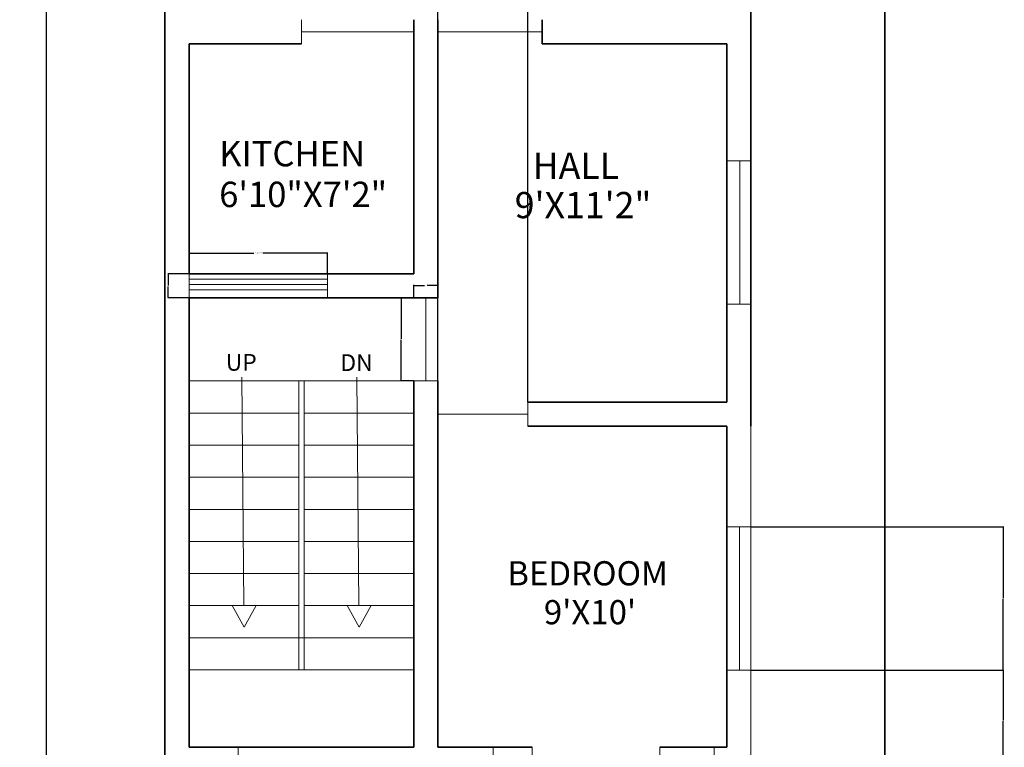
# Model space of a CAD drawing. Units: feet. Extents: x 2100 to 2836, y 2433 to 3396.
# Tile 6 of 12: x 2468 to 2836, y 2634 to 2906. Entities that reach past the tile are written whole.
import ezdxf

# ---------------------------------------------------------------- set-up
doc = ezdxf.new("R2010")
doc.units = ezdxf.units.FT
for name, color, linetype, lineweight in [('A-ANNO-DIMS', 2, 'Continuous', 18), ('A-ANNO-SYMB', 2, 'Continuous', 13), ('A-ANNO-TEXT', 7, 'Continuous', 18), ('A-ANNO-TTLB', 7, 'Continuous', 35), ('A-AREA-IDEN', 7, 'Continuous', 18), ('A-DOOR', 3, 'Continuous', 18), ('A-FLOR-STRS', 2, 'Continuous', 20), ('A-GLAZ', 4, 'Continuous', 18), ('A-WALL', 7, 'Continuous', 35), ('C-PROP', 8, 'Continuous', 18)]:
    doc.layers.add(name, color=color, linetype=linetype, lineweight=lineweight)
doc.styles.get("Standard").update_dxf_attribs({"font": 'arial.ttf'})
doc.dimstyles.get("Standard").update_dxf_attribs({"dimtxt": 0.18, "dimasz": 0.18, "dimexe": 0.18, "dimexo": 0.0625, "dimgap": 0.09, "dimtad": 0, "dimtih": 1, "dimtoh": 1, "dimdec": 4, "dimzin": 0, "dimdsep": 46, "dimtxsty": 'Standard', "dimcen": 0.09, "dimadec": 0, "dimazin": 0, "dimtfac": 1, "dimtdec": 4, "dimtofl": 0, "dimtmove": 0, "dimatfit": 3, "dimfxl": 1, "dimtolj": 1, "dimtzin": 0, "dimarcsym": 0})

# ---------------------------------------------------------------- blocks, each defined once
blk = doc.blocks.new('STAIR-RETURN-FLIGHT')
for p, q in [((84, 108), (0, 108)), ((41, 108), (41, 0)), ((43, 108), (43, 0)), ((41, 96), (0, 96)), ((84, 96), (43, 96)), ((41, 84), (0, 84)), ((84, 84), (43, 84)), ((41, 72), (0, 72)), ((84, 72), (43, 72)), ((41, 60), (0, 60)), ((84, 60), (43, 60)), ((41, 48), (0, 48)), ((84, 48), (43, 48)), ((41, 36), (0, 36)), ((84, 36), (43, 36)), ((41, 24), (0, 24)), ((84, 24), (43, 24)), ((84, 12), (0, 12)), ((84, 0), (0, 0))]:
    blk.add_line(p, q)
blk = doc.blocks.new('STAIR-DIRECTION')
for p, q in [((3.63, 93.38), (4.37, 8)), ((4.44, 0), (0, 8)), ((4.44, 0), (8.95, 8))]:
    blk.add_line(p, q)
blk = doc.blocks.new('WIN-KITCHEN')
for p, q in [((0, 9), (0, 0)), ((51.75, 9), (51.75, 0)), ((51.75, 7), (0, 7)), ((51.75, 5), (0, 5)), ((51.75, 3), (0, 3))]:
    blk.add_line(p, q)
blk = doc.blocks.new('DOOR-STAIR-HALL')
for p, q in [((4.5, 0), (4.5, 31.05)), ((9, 0), (0, 0))]:
    blk.add_line(p, q)
blk = doc.blocks.new('DOOR-PASSAGE')
for p, q in [((42, 0), (42, 9)), ((42, 4.5), (0, 4.5))]:
    blk.add_line(p, q)
blk = doc.blocks.new('DOOR-SLIDING-ENTRY')
for p, q in [((0, 9), (0, 0)), ((14.54, 9), (14.54, 0)), ((62.31, 9), (62.31, 0)), ((82.55, 9), (82.55, 0)), ((0, 4.5), (82.55, 4.5))]:
    blk.add_line(p, q)
blk = doc.blocks.new('*D22')
at = {"layer": 'A-ANNO-DIMS', "color": 0, "lineweight": -2, "transparency": 16777216}
for p, q in [((2530.95, 2810.87), (2530.95, 2818.75)), ((2531.13, 2818.57), (2555.12, 2818.57)), ((2582.52, 2818.57), (2558.52, 2818.57)), ((2582.7, 2810.87), (2582.7, 2818.75))]:
    blk.add_line(p, q, dxfattribs=at)
at = {"layer": 'A-ANNO-DIMS', "color": 0, "transparency": 16777216}
for points in [[(2531.13, 2818.6), (2531.13, 2818.54), (2530.95, 2818.57)], [(2582.52, 2818.6), (2582.52, 2818.54), (2582.7, 2818.57)]]:
    blk.add_solid(points, dxfattribs=at)
at = {"layer": 'Defpoints', "color": 0, "transparency": 16777216}
for p in [(2582.7, 2818.57), (2530.95, 2810.8), (2582.7, 2810.8)]:
    blk.add_point(p, dxfattribs=at)
at = {"layer": 'A-ANNO-DIMS', "color": 0, "transparency": 16777216, "insert": (2556.82, 2818.57), "char_height": 0.18, "attachment_point": 5}
blk.add_mtext('\\A1;KITCHEN WINDOW 52 TYP.', dxfattribs=at)
blk = doc.blocks.new('*D23')
at = {"layer": 'A-ANNO-DIMS', "color": 0, "lineweight": -2, "transparency": 16777216}
for p, q in [((2530.89, 2810.8), (2523.01, 2810.8)), ((2523.19, 2810.62), (2523.19, 2806.48)), ((2523.19, 2801.98), (2523.19, 2806.12)), ((2530.89, 2801.8), (2523.01, 2801.8))]:
    blk.add_line(p, q, dxfattribs=at)
at = {"layer": 'A-ANNO-DIMS', "color": 0, "transparency": 16777216}
for points in [[(2523.16, 2810.62), (2523.22, 2810.62), (2523.19, 2810.8)], [(2523.16, 2801.98), (2523.22, 2801.98), (2523.19, 2801.8)]]:
    blk.add_solid(points, dxfattribs=at)
at = {"layer": 'Defpoints', "color": 0, "transparency": 16777216}
for p in [(2523.19, 2810.8), (2530.95, 2810.8), (2530.95, 2801.8)]:
    blk.add_point(p, dxfattribs=at)
at = {"layer": 'A-ANNO-DIMS', "color": 0, "transparency": 16777216, "insert": (2523.19, 2806.3), "char_height": 0.18, "attachment_point": 5}
blk.add_mtext('\\A1;9 TYP.', dxfattribs=at)
blk = doc.blocks.new('*D36')
at = {"layer": 'A-ANNO-DIMS', "color": 0, "lineweight": -2, "transparency": 16777216}
for p, q in [((2614.89, 2801.8), (2610.11, 2801.8)), ((2610.29, 2801.62), (2610.29, 2786.46)), ((2610.29, 2770.94), (2610.29, 2786.1)), ((2614.89, 2770.76), (2610.11, 2770.76))]:
    blk.add_line(p, q, dxfattribs=at)
at = {"layer": 'A-ANNO-DIMS', "color": 0, "transparency": 16777216}
for points in [[(2610.26, 2801.62), (2610.32, 2801.62), (2610.29, 2801.8)], [(2610.26, 2770.94), (2610.32, 2770.94), (2610.29, 2770.76)]]:
    blk.add_solid(points, dxfattribs=at)
at = {"layer": 'Defpoints', "color": 0, "transparency": 16777216}
for p in [(2610.29, 2801.8), (2614.95, 2801.8), (2614.95, 2770.76)]:
    blk.add_point(p, dxfattribs=at)
at = {"layer": 'A-ANNO-DIMS', "color": 0, "transparency": 16777216, "insert": (2610.29, 2786.28), "char_height": 0.18, "attachment_point": 5}
blk.add_mtext('\\A1;HALL DOOR 31 TYP.', dxfattribs=at)
blk = doc.blocks.new('*D37')
at = {"layer": 'A-ANNO-DIMS', "color": 0, "lineweight": -2, "transparency": 16777216}
for p, q in [((2614.95, 2801.87), (2614.95, 2806.64)), ((2615.13, 2806.46), (2618.99, 2806.46)), ((2623.77, 2806.46), (2619.91, 2806.46)), ((2623.95, 2801.87), (2623.95, 2806.64))]:
    blk.add_line(p, q, dxfattribs=at)
at = {"layer": 'A-ANNO-DIMS', "color": 0, "transparency": 16777216}
for points in [[(2615.13, 2806.49), (2615.13, 2806.43), (2614.95, 2806.46)], [(2623.77, 2806.49), (2623.77, 2806.43), (2623.95, 2806.46)]]:
    blk.add_solid(points, dxfattribs=at)
at = {"layer": 'Defpoints', "color": 0, "transparency": 16777216}
for p in [(2623.95, 2806.46), (2614.95, 2801.8), (2623.95, 2801.8)]:
    blk.add_point(p, dxfattribs=at)
at = {"layer": 'A-ANNO-DIMS', "color": 0, "transparency": 16777216, "insert": (2619.45, 2806.46), "char_height": 0.18, "attachment_point": 5}
blk.add_mtext('\\A1;9 TYP.', dxfattribs=at)
blk = doc.blocks.new('*D43')
at = {"layer": 'A-ANNO-DIMS', "color": 0, "lineweight": -2, "transparency": 16777216}
for p, q in [((2521.89, 3321.8), (2477.52, 3321.8)), ((2477.7, 3321.62), (2477.7, 2929.96)), ((2477.7, 2537.94), (2477.7, 2929.6)), ((2521.89, 2537.76), (2477.52, 2537.76))]:
    blk.add_line(p, q, dxfattribs=at)
at = {"layer": 'A-ANNO-DIMS', "color": 0, "transparency": 16777216}
for points in [[(2477.67, 3321.62), (2477.73, 3321.62), (2477.7, 3321.8)], [(2477.67, 2537.94), (2477.73, 2537.94), (2477.7, 2537.76)]]:
    blk.add_solid(points, dxfattribs=at)
at = {"layer": 'Defpoints', "color": 0, "transparency": 16777216}
for p in [(2477.7, 3321.8), (2521.95, 3321.8), (2521.95, 2537.76)]:
    blk.add_point(p, dxfattribs=at)
at = {"layer": 'A-ANNO-DIMS', "color": 0, "transparency": 16777216, "insert": (2477.7, 2929.78), "char_height": 0.18, "attachment_point": 5}
blk.add_mtext('\\A1;784', dxfattribs=at)
blk = doc.blocks.new('*D57')
at = {"layer": 'A-ANNO-DIMS', "color": 0, "lineweight": -2, "transparency": 16777216}
for p, q in [((2741.01, 2662.65), (2835.49, 2662.65)), ((2835.31, 2662.47), (2835.31, 2643.91)), ((2835.31, 2624.98), (2835.31, 2643.54)), ((2741.01, 2624.8), (2835.49, 2624.8))]:
    blk.add_line(p, q, dxfattribs=at)
at = {"layer": 'A-ANNO-DIMS', "color": 0, "transparency": 16777216}
for points in [[(2835.28, 2662.47), (2835.34, 2662.47), (2835.31, 2662.65)], [(2835.28, 2624.98), (2835.34, 2624.98), (2835.31, 2624.8)]]:
    blk.add_solid(points, dxfattribs=at)
at = {"layer": 'Defpoints', "color": 0, "transparency": 16777216}
for p in [(2740.95, 2662.65), (2835.31, 2662.65), (2740.95, 2624.8)]:
    blk.add_point(p, dxfattribs=at)
at = {"layer": 'A-ANNO-DIMS', "color": 0, "transparency": 16777216, "insert": (2835.31, 2643.73), "char_height": 0.18, "attachment_point": 5}
blk.add_mtext('\\A1;37.845', dxfattribs=at)
blk = doc.blocks.new('*D58')
at = {"layer": 'A-ANNO-DIMS', "color": 0, "lineweight": -2, "transparency": 16777216}
for p, q in [((2741.01, 2716.27), (2835.49, 2716.27)), ((2835.31, 2716.09), (2835.31, 2689.64)), ((2835.31, 2662.83), (2835.31, 2689.28)), ((2741.01, 2662.65), (2835.49, 2662.65))]:
    blk.add_line(p, q, dxfattribs=at)
at = {"layer": 'A-ANNO-DIMS', "color": 0, "transparency": 16777216}
for points in [[(2835.28, 2716.09), (2835.34, 2716.09), (2835.31, 2716.27)], [(2835.28, 2662.83), (2835.34, 2662.83), (2835.31, 2662.65)]]:
    blk.add_solid(points, dxfattribs=at)
at = {"layer": 'Defpoints', "color": 0, "transparency": 16777216}
for p in [(2740.95, 2716.27), (2835.31, 2716.27), (2740.95, 2662.65)]:
    blk.add_point(p, dxfattribs=at)
at = {"layer": 'A-ANNO-DIMS', "color": 0, "transparency": 16777216, "insert": (2835.31, 2689.46), "char_height": 0.18, "attachment_point": 5}
blk.add_mtext('\\A1;53.62', dxfattribs=at)
blk = doc.blocks.new('*D62')
at = {"layer": 'A-ANNO-DIMS', "color": 0, "lineweight": -2, "transparency": 16777216}
for p, q in [((2623.95, 2762.87), (2623.95, 3396.05)), ((2624.13, 3395.87), (2640.32, 3395.87)), ((2657.43, 3395.87), (2641.24, 3395.87)), ((2657.61, 2762.87), (2657.61, 3396.05))]:
    blk.add_line(p, q, dxfattribs=at)
at = {"layer": 'A-ANNO-DIMS', "color": 0, "transparency": 16777216}
for points in [[(2624.13, 3395.9), (2624.13, 3395.84), (2623.95, 3395.87)], [(2657.43, 3395.9), (2657.43, 3395.84), (2657.61, 3395.87)]]:
    blk.add_solid(points, dxfattribs=at)
at = {"layer": 'Defpoints', "color": 0, "transparency": 16777216}
for p in [(2657.61, 3395.87), (2623.95, 2762.8), (2657.61, 2762.8)]:
    blk.add_point(p, dxfattribs=at)
at = {"layer": 'A-ANNO-DIMS', "color": 0, "transparency": 16777216, "insert": (2640.78, 3395.87), "char_height": 0.18, "attachment_point": 5}
blk.add_mtext('\\A1;33.665', dxfattribs=at)

msp = doc.modelspace()

# ---------------------------------------------------------------- linework, layer by layer
at = {"layer": 'A-ANNO-TTLB'}
msp.add_lwpolyline([(2144.0848, 3351.6245), (2791.0561, 3351.6245), (2791.0561, 2477.4373), (2144.0848, 2477.4373)], close=True, dxfattribs=at)
at = {"layer": 'A-DOOR'}
for p, q in [((2623.9476, 2901.3031), (2662.9476, 2901.3031)), ((2657.613, 2762.8031), (2657.613, 2753.8031)), ((2657.613, 2758.3031), (2623.9476, 2758.3031))]:
    msp.add_line(p, q, dxfattribs=at)
at = {"layer": 'A-GLAZ'}
for p, q in [((2731.9476, 2853.0255), (2740.9476, 2853.0255)), ((2736.8841, 2853.0255), (2736.8841, 2799.4059)), ((2731.9476, 2799.4059), (2740.9476, 2799.4059)), ((2731.9476, 2716.2675), (2740.9476, 2716.2675)), ((2736.662, 2716.2675), (2736.662, 2662.6479)), ((2731.9476, 2662.6479), (2740.9476, 2662.6479)), ((2549.3574, 2633.8031), (2549.3574, 2624.8031))]:
    msp.add_line(p, q, dxfattribs=at)
at = {"layer": 'A-WALL'}
for p, q in [((2521.9476, 2593.755), (2521.9476, 3321.8031)), ((2740.9476, 2987.2733), (2740.9476, 2891.1053)), ((2614.9476, 2810.8031), (2614.9476, 2905.8031)), ((2623.9476, 2801.8031), (2623.9476, 2905.8031)), ((2662.9476, 2905.8031), (2662.9476, 2896.8031)), ((2530.9476, 2810.8031), (2530.9476, 2896.8031)), ((2572.9476, 2896.8031), (2530.9476, 2896.8031)), ((2662.9476, 2896.8031), (2731.9476, 2896.8031)), ((2731.9476, 2896.8031), (2731.9476, 2762.8031)), ((2740.9476, 2896.8031), (2740.9476, 2753.8031)), ((2614.9476, 2810.8031), (2530.9476, 2810.8031)), ((2623.9476, 2801.8031), (2530.9476, 2801.8031)), ((2530.9476, 2633.8031), (2530.9476, 2801.8031)), ((2614.9476, 2753.8031), (2614.9476, 2770.755)), ((2614.9476, 2770.755), (2614.9476, 2633.8031)), ((2623.9476, 2762.8031), (2623.9476, 2770.755)), ((2623.9476, 2770.755), (2623.9476, 2753.8031)), ((2731.9476, 2762.8031), (2657.613, 2762.8031)), ((2731.9476, 2762.8031), (2705.3766, 2762.8031)), ((2623.9476, 2753.8031), (2623.9476, 2633.8031)), ((2731.9476, 2753.8031), (2657.613, 2753.8031)), ((2731.9476, 2753.8031), (2705.3766, 2753.8031)), ((2731.9476, 2753.8031), (2731.9476, 2633.8031)), ((2614.9476, 2633.8031), (2530.9476, 2633.8031)), ((2659.1783, 2633.8031), (2623.9476, 2633.8031)), ((2731.9476, 2633.8031), (2706.9394, 2633.8031))]:
    msp.add_line(p, q, dxfattribs=at)
at = {"layer": 'C-PROP'}
msp.add_line((2740.9476, 2753.8031), (2740.9476, 2537.755), dxfattribs=at)

# ---------------------------------------------------------------- block references
at = {"layer": 'A-ANNO-SYMB'}
for p in [(2547.0789, 2678.7553), (2590.0789, 2678.7553)]:
    msp.add_blockref('STAIR-DIRECTION', p, dxfattribs=at)
at = {"layer": 'A-DOOR', "rotation": 180}
msp.add_blockref('DOOR-PASSAGE', (2614.9476, 2905.8031), dxfattribs=at)
at = {"layer": 'A-DOOR'}
for name, p in [('DOOR-STAIR-HALL', (2614.9476, 2770.755)), ('DOOR-SLIDING-ENTRY', (2644.6339, 2624.8031))]:
    msp.add_blockref(name, p, dxfattribs=at)
at = {"layer": 'A-FLOR-STRS'}
msp.add_blockref('STAIR-RETURN-FLIGHT', (2530.9476, 2662.755), dxfattribs=at)
at = {"layer": 'A-GLAZ'}
msp.add_blockref('WIN-KITCHEN', (2530.9476, 2801.8031), dxfattribs=at)

# ---------------------------------------------------------------- texts
at = {"layer": 'A-ANNO-TEXT'}
for s, p in [('UP', (2544.6814, 2774.568)), ('DN', (2587.5335, 2774.4717))]:
    msp.add_text(s, height=6.26655, dxfattribs=at).set_placement(p)
at = {"layer": 'A-AREA-IDEN'}
for s, height, p in [('KITCHEN', 9.48042, (2542.22, 2850.9877)), ('HALL', 9.79205, (2659.3786, 2846.3015)), ('6\'10"X7\'2"', 9.48042, (2542.22, 2835.7582)), ('9\'X11\'2"', 9.79205, (2652.692, 2831.5994)), ('BEDROOM', 9.04706, (2649.887, 2694.3287)), ("9'X10'", 9.04706, (2663.5727, 2679.7954))]:
    msp.add_text(s, height=height, dxfattribs=at).set_placement(p)

# ---------------------------------------------------------------- dimensions: what is measured, and where the dimension line sits
at = {"layer": 'A-ANNO-DIMS'}
dim = msp.add_linear_dim(base=(2657.613, 3395.8745), p1=(2623.9476, 2762.8031), p2=(2657.613, 2762.8031), dimstyle='Standard', override={"dimdec": 3, "dimlfac": 1, "dimrnd": 0, "dimzin": 0, "dimdsep": 46, "dimlunit": 2}, dxfattribs=at)
dim.commit()
dim.dimension.update_dxf_attribs({"geometry": '*D62', "text_midpoint": (2640.7803, 3395.8745)})
for base, p1, p2, override, picture, middle in [((2477.6976, 3321.8031), (2521.9476, 2537.755), (2521.9476, 3321.8031), {"dimdec": 0, "dimlfac": 1, "dimrnd": 0, "dimzin": 0, "dimdsep": 46, "dimlunit": 2}, '*D43', (2477.6976, 2929.7791)), ((2835.3061, 2716.2675), (2740.9476, 2662.6479), (2740.9476, 2716.2675), {"dimdec": 2, "dimlfac": 1, "dimrnd": 0, "dimzin": 0, "dimdsep": 46, "dimlunit": 2}, '*D58', (2835.3061, 2689.4577)), ((2835.3061, 2662.6479), (2740.9476, 2624.8031), (2740.9476, 2662.6479), {"dimdec": 3, "dimlfac": 1, "dimrnd": 0, "dimzin": 0, "dimdsep": 46, "dimlunit": 2}, '*D57', (2835.3061, 2643.7255))]:
    dim = msp.add_linear_dim(base=base, p1=p1, p2=p2, angle=90, dimstyle='Standard', override=override, dxfattribs=at)
    dim.commit()
    dim.dimension.update_dxf_attribs({"geometry": picture, "text_midpoint": middle})
for base, p1, p2, text, picture, middle in [((2582.6972, 2818.5655), (2530.9476, 2810.8031), (2582.6972, 2810.8031), 'KITCHEN WINDOW <> TYP.', '*D22', (2556.8224, 2818.5655)), ((2623.9476, 2806.4603), (2614.9476, 2801.8031), (2623.9476, 2801.8031), '<> TYP.', '*D37', (2619.4476, 2806.4603))]:
    dim = msp.add_linear_dim(base=base, p1=p1, p2=p2, text=text, dimstyle='Standard', override={"dimdec": 0, "dimlfac": 1, "dimrnd": 0, "dimzin": 0, "dimdsep": 46, "dimlunit": 2}, dxfattribs=at)
    dim.commit()
    dim.dimension.update_dxf_attribs({"geometry": picture, "text_midpoint": middle})
for base, p1, p2, text, picture, middle in [((2523.1852, 2810.8031), (2530.9476, 2801.8031), (2530.9476, 2810.8031), '<> TYP.', '*D23', (2523.1852, 2806.3031)), ((2610.2904, 2801.8031), (2614.9476, 2770.755), (2614.9476, 2801.8031), 'HALL DOOR <> TYP.', '*D36', (2610.2904, 2786.2791))]:
    dim = msp.add_linear_dim(base=base, p1=p1, p2=p2, angle=90, text=text, dimstyle='Standard', override={"dimdec": 0, "dimlfac": 1, "dimrnd": 0, "dimzin": 0, "dimdsep": 46, "dimlunit": 2}, dxfattribs=at)
    dim.commit()
    dim.dimension.update_dxf_attribs({"geometry": picture, "text_midpoint": middle})

doc.saveas('drawing.dxf')
